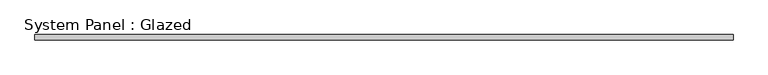
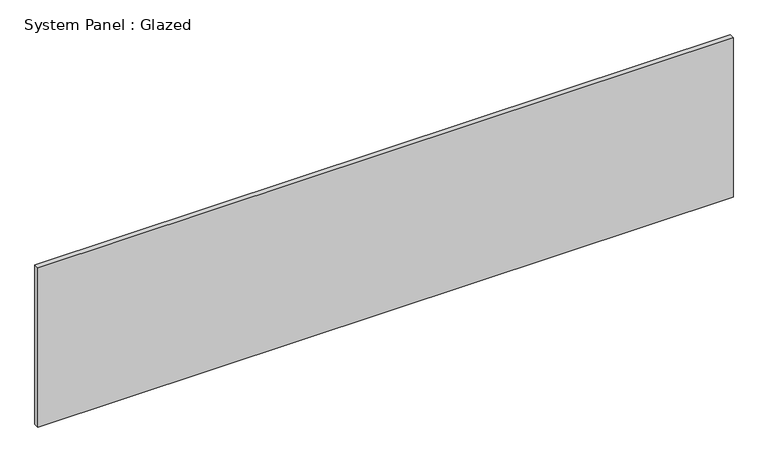
"""IFC4 building model written with IfcOpenShell, lengths in millimetres: plate geometry, System Panel : Glazed."""

from ifc_helpers import new_model, si_unit, origin, origin_with_axes, place, context, project, spatial, polyline, outline, extrude, source, transform, mapped, element, save


def system_panel_glazed_59f99603(model_context):
    return source(origin(), model_context, "Body", "SweptSolid", [
        extrude(outline(polyline([(1675.8227273, 19.05), (-1675.8227273, 19.05), (-1675.8227273, 44.45), (1675.8227273, 44.45), (1675.8227273, 19.05)])), origin_with_axes(), (0.0, 0.0, 1.0), 812.8),
    ])


if __name__ == "__main__":
    model = new_model("IFC4")
    model_context = context("Model", 3, world=origin())
    ifc_project = project(units=[si_unit("LENGTHUNIT", "METRE", prefix="MILLI")], contexts=[model_context])
    site = spatial("IfcSite", under=ifc_project)
    building = spatial("IfcBuilding", under=site)
    placement = place(None, origin())
    system_panel_glazed_shape = system_panel_glazed_59f99603(model_context)
    element("IfcPlate", 1, ObjectType="System Panel : Glazed", at=placement, inside=building, context=model_context, shape_type="MappedRepresentation", body=[
        mapped(system_panel_glazed_shape, transform((0.0, 0.0, 0.0), x_axis=(1.0, 0.0, 0.0), y_axis=(0.0, 1.0, 0.0), z_axis=(0.0, 0.0, 1.0))),
    ])
    save(model, "model.ifc")

# Revit data of these elements
# Type "System Panel : Glazed"
#   Construction Type Id = "GSP4R"
#   Analytic Construction = "1/8 in Pilkington single glazing"
#   Visual Light Transmittance = 0.9
#   Solar Heat Gain Coefficient = 0.86
#   Heat Transfer Coefficient (U) = 1.18115 BTU/(h·ft²·°F)
#   Define Thermal Properties by = 1
# Element 1 (IfcPlate, "System Panel : Glazed")
#   Materials on its faces: "Glass"
# Materials
#   "Glass": class "Glass", colour RGB 0 128 192, transparency 0.75, Description = "Soda Lime Glass", Cost = 0
